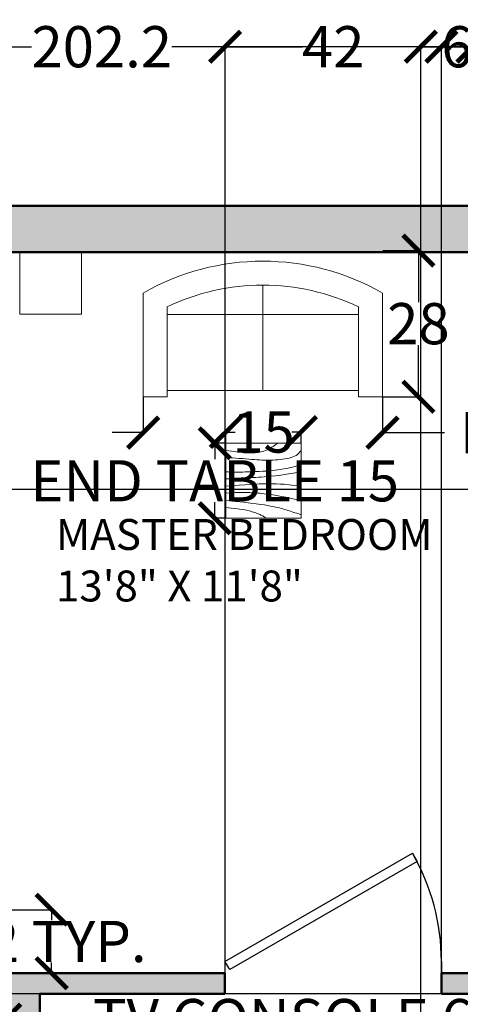
# Model space of a CAD drawing. Units: inches. Extents: x -30 to 744, y -375 to 57.
# Tile 4 of 8: x 116 to 202, y -134 to 57. Entities that reach past the tile are written whole.
import ezdxf

# ---------------------------------------------------------------- set-up
doc = ezdxf.new("R2010")
doc.units = ezdxf.units.IN
doc.header["$MEASUREMENT"] = 0
for name, color, linetype, lineweight in [('A-ANNO-DIMS', 2, 'Continuous', 18), ('A-AREA-IDEN', 7, 'Continuous', 25), ('A-DOOR', 3, 'Continuous', 25), ('A-FURN', 8, 'Continuous', 18), ('A-WALL', 7, 'Continuous', 50)]:
    doc.layers.add(name, color=color, linetype=linetype, lineweight=lineweight)
doc.layers.add('A-WALL-PATT', color=251, linetype='Continuous', lineweight=13, true_color=0x636466)
doc.styles.get("Standard").update_dxf_attribs({"font": 'arial.ttf'})
doc.dimstyles.get("Standard").update_dxf_attribs({"dimtxt": 8, "dimasz": 6, "dimexe": 0.18, "dimexo": 0.0625, "dimgap": 0.09, "dimtad": 0, "dimtih": 1, "dimtoh": 1, "dimdec": 0, "dimzin": 0, "dimdsep": 46, "dimlunit": 4, "dimtxsty": 'Standard', "dimblk": 'ARCHTICK', "dimcen": 0.09, "dimadec": 0, "dimazin": 0, "dimtfac": 1, "dimtdec": 0, "dimtofl": 0, "dimtmove": 0, "dimatfit": 1, "dimldrblk": 'ARCHTICK', "dimfxl": 1, "dimtolj": 1, "dimtzin": 0, "dimarcsym": 0})

# ---------------------------------------------------------------- blocks, each defined once
blk = doc.blocks.new('*U2')
for p, q in [((0, 0), (0, -6)), ((40, 0), (40, -6))]:
    blk.add_line(p, q)
blk.add_lwpolyline([(0, 0), (34.64, 20), (35.52, 18.48), (0.87, -1.52)], close=True)
blk.add_arc((0, 0), 40, 0, 30)
blk = doc.blocks.new('Table - Square Woodgrain 42 x 42 in.')
blk.add_line((0, -42), (42, -42))
for points in [[(0, -4), (1.704, -4.2172), (3.2358, -4.4188), (4.615, -4.604), (5.8615, -4.7721), (6.9951, -4.9224), (8.0357, -5.0541), (9.0031, -5.1667), (9.9171, -5.2594), (10.7951, -5.3316), (11.6445, -5.3836), (12.4702, -5.4157), (13.277, -5.4283), (14.0698, -5.4217), (14.8535, -5.3964), (15.6331, -5.3526), (16.4133, -5.2908), (17.1986, -5.2103), (17.9913, -5.1062), (18.793, -4.9727), (19.6056, -4.8038), (20.4307, -4.5937), (21.2701, -4.3365), (22.1256, -4.0262), (22.9989, -3.6571), (23.888, -3.2272), (24.7756, -2.7516), (25.6408, -2.2491), (26.4624, -1.7387), (27.2195, -1.2395), (27.891, -0.7703), (28.456, -0.3501), (28.8934, 0.002)], [(0, -42), (0, 0), (42, 0), (42, -42)], [(0, -8), (1.8203, -8.1001), (3.6741, -8.2149), (5.5411, -8.3408), (7.4011, -8.4741), (9.2339, -8.6112), (11.0193, -8.7484), (12.7371, -8.8821), (14.3671, -9.0086), (15.8954, -9.1246), (17.3337, -9.2278), (18.6997, -9.3159), (20.0116, -9.387), (21.2871, -9.4389), (22.5442, -9.4696), (23.8008, -9.477), (25.0749, -9.459), (26.3791, -9.4137), (27.7049, -9.3403), (29.0383, -9.2382), (30.3655, -9.1068), (31.6728, -8.9455), (32.9461, -8.7535), (34.1717, -8.5304), (35.3358, -8.2756), (36.4268, -7.9863), (37.443, -7.6521), (38.3849, -7.2603), (39.253, -6.7986), (40.048, -6.2542), (40.7705, -5.6147), (41.421, -4.8674), (42, -4)], [(42, -12), (39.1784, -12.8621), (36.4519, -13.5654), (33.8246, -14.1294), (31.3004, -14.5731), (28.8832, -14.9161), (26.577, -15.1775), (24.3858, -15.3768), (22.3136, -15.5332), (20.3622, -15.6632), (18.5254, -15.7718), (16.7947, -15.8612), (15.1618, -15.9338), (13.6183, -15.9916), (12.1558, -16.0369), (10.7659, -16.0718), (9.4403, -16.0987), (8.1703, -16.1191), (6.9461, -16.1325), (5.7577, -16.1377), (4.595, -16.1335), (3.4479, -16.1188), (2.3064, -16.0924), (1.1604, -16.0532), (0, -16)], [(42, -16), (37.6529, -16.7365), (33.8802, -17.329), (30.6179, -17.7961), (27.8015, -18.1561), (25.3668, -18.4275), (23.2497, -18.6288), (21.3859, -18.7785), (19.7111, -18.8949), (18.1693, -18.9939), (16.7375, -19.0795), (15.401, -19.1534), (14.1449, -19.217), (12.9544, -19.2717), (11.8148, -19.3191), (10.7113, -19.3606), (9.6291, -19.3976), (8.5534, -19.4323), (7.47, -19.4689), (6.3643, -19.5122), (5.222, -19.5672), (4.0288, -19.6386), (2.7703, -19.7313), (1.4321, -19.8501), (0, -20)], [(0, -24), (3.9243, -23.6805), (7.4766, -23.4138), (10.6891, -23.1954), (13.5943, -23.0205), (16.2247, -22.8847), (18.6125, -22.7832), (20.7903, -22.7116), (22.7903, -22.6651), (24.6563, -22.642), (26.4764, -22.6507), (28.35, -22.7024), (30.3766, -22.8084), (32.6555, -22.98), (35.2861, -23.2283), (38.3678, -23.5645), (42, -24)], [(42, -32), (37.392, -31.017), (33.4585, -30.2231), (30.1291, -29.5949), (27.3334, -29.109), (25.0009, -28.742), (23.0612, -28.4707), (21.4439, -28.2716), (20.0786, -28.1215), (18.8998, -28.0002), (17.8609, -27.9014), (16.9206, -27.8219), (16.0371, -27.7588), (15.1691, -27.709), (14.2748, -27.6693), (13.3128, -27.6368), (12.2415, -27.6083), (11.0295, -27.5824), (9.6867, -27.5643), (8.233, -27.5608), (6.6884, -27.5787), (5.0728, -27.6248), (3.4062, -27.7058), (1.7086, -27.8286), (0, -28)], [(0, -32), (5.4026, -32.5358), (9.9494, -33.019), (13.7424, -33.4553), (16.8834, -33.8505), (19.4743, -34.2106), (21.6171, -34.5413), (23.4136, -34.8486), (24.9657, -35.1382), (26.3614, -35.4156), (27.6332, -35.6841), (28.7995, -35.9467), (29.8788, -36.2064), (30.8897, -36.4661), (31.8507, -36.7288), (32.7802, -36.9973), (33.6968, -37.2747), (34.6175, -37.5635), (35.5531, -37.8651), (36.5128, -38.1805), (37.506, -38.5108), (38.5421, -38.8568), (39.6302, -39.2197), (40.7797, -39.6004), (42, -40)], [(0, -36), (3.0098, -36.2857), (5.5354, -36.5643), (7.6368, -36.8359), (9.374, -37.1009), (10.807, -37.3597), (11.9957, -37.6126), (13.0002, -37.8599), (13.8804, -38.102), (14.6874, -38.3393), (15.4365, -38.5729), (16.1338, -38.8041), (16.7858, -39.0341), (17.3987, -39.264), (17.9787, -39.4952), (18.5322, -39.7288), (19.0655, -39.9662), (19.5832, -40.2081), (20.0842, -40.4544), (20.5657, -40.7046), (21.0249, -40.9581), (21.459, -41.2144), (21.8653, -41.4731), (22.2409, -41.7335), (22.5831, -41.9951)]]:
    blk.add_lwpolyline(points)
blk = doc.blocks.new('Sofa - Roundback Loveseat 5 ft.')
for p, q in [((0, -32.44198), (0, -5.99998)), ((-24, -33.99998), (-24, -11.46958)), ((24.00004, -33.99998), (24.00004, -11.46958)), ((-23.9998, -13.38178), (23.99986, -13.38178)), ((-24, -32.44198), (24.00004, -32.44198))]:
    blk.add_line(p, q)
for points in [[(-24, -33.99998), (-30, -33.99998), (-30, -7.99998)], [(30.00004, -7.99998), (30.00004, -33.99998), (24.00004, -33.99998)]]:
    blk.add_lwpolyline(points)
for centre, radius, start, end in [((0, -60.24998), 60.24998, 60.13715, 119.8628), ((0, -61.38438), 55.38444, 64.32083, 115.6792)]:
    blk.add_arc(centre, radius, start, end)
blk = doc.blocks.new('NIGHTSTAND-12IN')
blk.add_lwpolyline([(0, 12), (0, 0), (12, 0), (12, 12)], close=True)
blk = doc.blocks.new('_ArchTick')
at = {"color": 0, "linetype": 'ByBlock', "const_width": 0.15}
blk.add_lwpolyline([(-0.5, -0.5), (0.5, 0.5)], dxfattribs=at)
blk = doc.blocks.new('*D44')
at = {"layer": 'A-ANNO-DIMS', "color": 0, "lineweight": -2, "transparency": 16777216}
for p, q in [((53.6, -128.37), (53.6, -137.48)), ((113.6, -128.37), (113.6, -137.48)), ((53.6, -137.3), (47.6, -137.3)), ((113.6, -137.3), (125.6, -137.3))]:
    blk.add_line(p, q, dxfattribs=at)
at = {"layer": 'Defpoints', "color": 0, "transparency": 16777216}
for p in [(53.6, -128.3), (113.6, -128.3), (113.6, -137.3)]:
    blk.add_point(p, dxfattribs=at)
at = {"layer": 'A-ANNO-DIMS', "color": 0, "lineweight": -2, "transparency": 16777216, "xscale": 6, "yscale": 6, "zscale": 6}
blk.add_blockref('_ArchTick', (53.6, -137.3), dxfattribs=at)
at = {"layer": 'A-ANNO-DIMS', "color": 0, "lineweight": -2, "transparency": 16777216, "xscale": 6, "yscale": 6, "zscale": 6, "rotation": 180}
blk.add_blockref('_ArchTick', (113.6, -137.3), dxfattribs=at)
at = {"layer": 'A-ANNO-DIMS', "color": 0, "transparency": 16777216, "insert": (182.83, -137.3), "char_height": 8, "attachment_point": 5}
blk.add_mtext('\\A1;TV CONSOLE 60 TYP.', dxfattribs=at)
blk = doc.blocks.new('*D45')
at = {"layer": 'A-ANNO-DIMS', "color": 0, "lineweight": -2, "transparency": 16777216}
for p, q in [((113.66, -115.96), (122.78, -115.96)), ((122.6, -115.96), (122.6, -118.02)), ((122.6, -128.3), (122.6, -126.24)), ((113.66, -128.3), (122.78, -128.3))]:
    blk.add_line(p, q, dxfattribs=at)
at = {"layer": 'Defpoints', "color": 0, "transparency": 16777216}
for p in [(113.6, -115.96), (122.6, -115.96), (113.6, -128.3)]:
    blk.add_point(p, dxfattribs=at)
at = {"layer": 'A-ANNO-DIMS', "color": 0, "lineweight": -2, "transparency": 16777216, "xscale": 6, "yscale": 6, "zscale": 6}
for p, rotation in [((122.6, -115.96), 90), ((122.6, -128.3), 270)]:
    blk.add_blockref('_ArchTick', p, dxfattribs=dict(at, rotation=rotation))
at = {"layer": 'A-ANNO-DIMS', "color": 0, "transparency": 16777216, "insert": (122.6, -122.13), "char_height": 8, "attachment_point": 5}
blk.add_mtext('\\A1;12 TYP.', dxfattribs=at)
blk = doc.blocks.new('*D54')
at = {"layer": 'A-ANNO-DIMS', "color": 0, "lineweight": -2, "transparency": 16777216}
for p, q in [((156.36, -25.4), (154.06, -25.4)), ((154.24, -25.4), (154.24, -28.5)), ((154.24, -39.96), (154.24, -36.85)), ((156.36, -39.96), (154.06, -39.96))]:
    blk.add_line(p, q, dxfattribs=at)
at = {"layer": 'Defpoints', "color": 0, "transparency": 16777216}
for p in [(154.24, -25.4), (156.42, -25.4), (156.42, -39.96)]:
    blk.add_point(p, dxfattribs=at)
at = {"layer": 'A-ANNO-DIMS', "color": 0, "lineweight": -2, "transparency": 16777216, "xscale": 6, "yscale": 6, "zscale": 6}
for p, rotation in [((154.24, -25.4), 90), ((154.24, -39.96), 270)]:
    blk.add_blockref('_ArchTick', p, dxfattribs=dict(at, rotation=rotation))
at = {"layer": 'A-ANNO-DIMS', "color": 0, "transparency": 16777216, "insert": (154.24, -32.68), "char_height": 8, "attachment_point": 5}
blk.add_mtext('\\A1;END TABLE 15', dxfattribs=at)
blk = doc.blocks.new('*D55')
at = {"layer": 'A-ANNO-DIMS', "color": 0, "lineweight": -2, "transparency": 16777216}
for p, q in [((156.42, -25.33), (156.42, -23.03)), ((156.42, -23.21), (158.23, -23.21)), ((170.99, -23.21), (169.18, -23.21)), ((170.99, -25.33), (170.99, -23.03))]:
    blk.add_line(p, q, dxfattribs=at)
at = {"layer": 'Defpoints', "color": 0, "transparency": 16777216}
for p in [(170.99, -23.21), (156.42, -25.4), (170.99, -25.4)]:
    blk.add_point(p, dxfattribs=at)
at = {"layer": 'A-ANNO-DIMS', "color": 0, "lineweight": -2, "transparency": 16777216, "xscale": 6, "yscale": 6, "zscale": 6, "rotation": 180}
blk.add_blockref('_ArchTick', (156.42, -23.21), dxfattribs=at)
at = {"layer": 'A-ANNO-DIMS', "color": 0, "lineweight": -2, "transparency": 16777216, "xscale": 6, "yscale": 6, "zscale": 6}
blk.add_blockref('_ArchTick', (170.99, -23.21), dxfattribs=at)
at = {"layer": 'A-ANNO-DIMS', "color": 0, "transparency": 16777216, "insert": (163.71, -23.21), "char_height": 8, "attachment_point": 5}
blk.add_mtext('\\A1;15', dxfattribs=at)
blk = doc.blocks.new('*D56')
at = {"layer": 'A-ANNO-DIMS', "color": 0, "lineweight": -2, "transparency": 16777216}
for p, q in [((140.35, -16.43), (140.35, -23.51)), ((186.8, -16.43), (186.8, -23.51)), ((140.35, -23.33), (134.35, -23.33)), ((186.8, -23.33), (198.8, -23.33))]:
    blk.add_line(p, q, dxfattribs=at)
at = {"layer": 'Defpoints', "color": 0, "transparency": 16777216}
for p in [(140.35, -16.36), (186.8, -16.36), (186.8, -23.33)]:
    blk.add_point(p, dxfattribs=at)
at = {"layer": 'A-ANNO-DIMS', "color": 0, "lineweight": -2, "transparency": 16777216, "xscale": 6, "yscale": 6, "zscale": 6}
blk.add_blockref('_ArchTick', (140.35, -23.33), dxfattribs=at)
at = {"layer": 'A-ANNO-DIMS', "color": 0, "lineweight": -2, "transparency": 16777216, "xscale": 6, "yscale": 6, "zscale": 6, "rotation": 180}
blk.add_blockref('_ArchTick', (186.8, -23.33), dxfattribs=at)
at = {"layer": 'A-ANNO-DIMS', "color": 0, "transparency": 16777216, "insert": (235.5, -23.33), "char_height": 8, "attachment_point": 5}
blk.add_mtext('\\A1;LOVESEAT 46', dxfattribs=at)
blk = doc.blocks.new('*D57')
at = {"layer": 'A-ANNO-DIMS', "color": 0, "lineweight": -2, "transparency": 16777216}
for p, q in [((186.86, 12.03), (193.95, 12.03)), ((193.77, 12.03), (193.77, 2.01)), ((193.77, -16.36), (193.77, -6.34)), ((186.86, -16.36), (193.95, -16.36))]:
    blk.add_line(p, q, dxfattribs=at)
at = {"layer": 'Defpoints', "color": 0, "transparency": 16777216}
for p in [(186.8, 12.03), (193.77, 12.03), (186.8, -16.36)]:
    blk.add_point(p, dxfattribs=at)
at = {"layer": 'A-ANNO-DIMS', "color": 0, "lineweight": -2, "transparency": 16777216, "xscale": 6, "yscale": 6, "zscale": 6}
for p, rotation in [((193.77, 12.03), 90), ((193.77, -16.36), 270)]:
    blk.add_blockref('_ArchTick', p, dxfattribs=dict(at, rotation=rotation))
at = {"layer": 'A-ANNO-DIMS', "color": 0, "transparency": 16777216, "insert": (193.77, -2.17), "char_height": 8, "attachment_point": 5}
blk.add_mtext('\\A1;28', dxfattribs=at)
blk = doc.blocks.new('*D63')
at = {"layer": 'A-ANNO-DIMS', "color": 0, "lineweight": -2, "transparency": 16777216}
for p, q in [((542.17, -132.3), (-16.61, -132.3)), ((-16.43, -132.3), (-16.43, -157.12)), ((-16.43, -190.3), (-16.43, -165.47)), ((542.17, -190.3), (-16.61, -190.3))]:
    blk.add_line(p, q, dxfattribs=at)
at = {"layer": 'Defpoints', "color": 0, "transparency": 16777216}
for p in [(-16.43, -132.3), (542.24, -132.3), (542.24, -190.3)]:
    blk.add_point(p, dxfattribs=at)
at = {"layer": 'A-ANNO-DIMS', "color": 0, "lineweight": -2, "transparency": 16777216, "xscale": 6, "yscale": 6, "zscale": 6}
for p, rotation in [((-16.43, -132.3), 90), ((-16.43, -190.3), 270)]:
    blk.add_blockref('_ArchTick', p, dxfattribs=dict(at, rotation=rotation))
at = {"layer": 'A-ANNO-DIMS', "color": 0, "transparency": 16777216, "insert": (-16.43, -161.3), "char_height": 8, "attachment_point": 5}
blk.add_mtext('\\A1;58', dxfattribs=at)
blk = doc.blocks.new('*D66')
at = {"layer": 'A-ANNO-DIMS', "color": 0, "lineweight": -2, "transparency": 16777216}
for p, q in [((156.24, -128.23), (156.24, 51.78)), ((198.24, -128.23), (198.24, 51.78)), ((156.24, 51.6), (171.3, 51.6)), ((198.24, 51.6), (183.18, 51.6))]:
    blk.add_line(p, q, dxfattribs=at)
at = {"layer": 'Defpoints', "color": 0, "transparency": 16777216}
for p in [(198.24, 51.6), (156.24, -128.3), (198.24, -128.3)]:
    blk.add_point(p, dxfattribs=at)
at = {"layer": 'A-ANNO-DIMS', "color": 0, "lineweight": -2, "transparency": 16777216, "xscale": 6, "yscale": 6, "zscale": 6, "rotation": 180}
blk.add_blockref('_ArchTick', (156.24, 51.6), dxfattribs=at)
at = {"layer": 'A-ANNO-DIMS', "color": 0, "lineweight": -2, "transparency": 16777216, "xscale": 6, "yscale": 6, "zscale": 6}
blk.add_blockref('_ArchTick', (198.24, 51.6), dxfattribs=at)
at = {"layer": 'A-ANNO-DIMS', "color": 0, "transparency": 16777216, "insert": (177.24, 51.6), "char_height": 8, "attachment_point": 5}
blk.add_mtext('\\A1;42', dxfattribs=at)
blk = doc.blocks.new('*D69')
at = {"layer": 'A-ANNO-DIMS', "color": 0, "lineweight": -2, "transparency": 16777216}
for p, q in [((31.24, 20.77), (31.24, 51.78)), ((233.43, 20.77), (233.43, 51.78)), ((31.24, 51.6), (118.72, 51.6)), ((233.43, 51.6), (145.95, 51.6))]:
    blk.add_line(p, q, dxfattribs=at)
at = {"layer": 'Defpoints', "color": 0, "transparency": 16777216}
for p in [(233.43, 51.6), (31.24, 20.7), (233.43, 20.7)]:
    blk.add_point(p, dxfattribs=at)
at = {"layer": 'A-ANNO-DIMS', "color": 0, "lineweight": -2, "transparency": 16777216, "xscale": 6, "yscale": 6, "zscale": 6, "rotation": 180}
blk.add_blockref('_ArchTick', (31.24, 51.6), dxfattribs=at)
at = {"layer": 'A-ANNO-DIMS', "color": 0, "lineweight": -2, "transparency": 16777216, "xscale": 6, "yscale": 6, "zscale": 6}
blk.add_blockref('_ArchTick', (233.43, 51.6), dxfattribs=at)
at = {"layer": 'A-ANNO-DIMS', "color": 0, "transparency": 16777216, "insert": (132.33, 51.6), "char_height": 8, "attachment_point": 5}
blk.add_mtext('\\A1;202.2', dxfattribs=at)
blk = doc.blocks.new('*D73')
at = {"layer": 'A-ANNO-DIMS', "color": 0, "lineweight": -2, "transparency": 16777216}
for p, q in [((194.24, -330.23), (194.24, 51.78)), ((230.24, -330.23), (230.24, 51.78)), ((194.24, 51.6), (206.42, 51.6)), ((230.24, 51.6), (218.05, 51.6))]:
    blk.add_line(p, q, dxfattribs=at)
at = {"layer": 'Defpoints', "color": 0, "transparency": 16777216}
for p in [(230.24, 51.6), (194.24, -330.3), (230.24, -330.3)]:
    blk.add_point(p, dxfattribs=at)
at = {"layer": 'A-ANNO-DIMS', "color": 0, "lineweight": -2, "transparency": 16777216, "xscale": 6, "yscale": 6, "zscale": 6, "rotation": 180}
blk.add_blockref('_ArchTick', (194.24, 51.6), dxfattribs=at)
at = {"layer": 'A-ANNO-DIMS', "color": 0, "lineweight": -2, "transparency": 16777216, "xscale": 6, "yscale": 6, "zscale": 6}
blk.add_blockref('_ArchTick', (230.24, 51.6), dxfattribs=at)
at = {"layer": 'A-ANNO-DIMS', "color": 0, "transparency": 16777216, "insert": (212.24, 51.6), "char_height": 8, "attachment_point": 5}
blk.add_mtext('\\A1;36', dxfattribs=at)
blk = doc.blocks.new('*D75')
at = {"layer": 'A-ANNO-DIMS', "color": 0, "lineweight": -2, "transparency": 16777216}
for p, q in [((40.3, 11.7), (662.32, 11.7)), ((662.14, 11.7), (662.14, -7.12)), ((662.14, -34.3), (662.14, -15.47)), ((40.3, -34.3), (662.32, -34.3))]:
    blk.add_line(p, q, dxfattribs=at)
at = {"layer": 'Defpoints', "color": 0, "transparency": 16777216}
for p in [(40.24, 11.7), (662.14, 11.7), (40.24, -34.3)]:
    blk.add_point(p, dxfattribs=at)
at = {"layer": 'A-ANNO-DIMS', "color": 0, "lineweight": -2, "transparency": 16777216, "xscale": 6, "yscale": 6, "zscale": 6}
for p, rotation in [((662.14, 11.7), 90), ((662.14, -34.3), 270)]:
    blk.add_blockref('_ArchTick', p, dxfattribs=dict(at, rotation=rotation))
at = {"layer": 'A-ANNO-DIMS', "color": 0, "transparency": 16777216, "insert": (662.14, -11.3), "char_height": 8, "attachment_point": 5}
blk.add_mtext('\\A1;46', dxfattribs=at)
blk = doc.blocks.new('*D86')
at = {"layer": 'A-ANNO-DIMS', "color": 0, "lineweight": -2, "transparency": 16777216}
for p, q in [((198.24, -128.23), (198.24, 51.78)), ((204.24, -128.23), (204.24, 51.78)), ((198.24, 51.6), (198.5, 51.6)), ((204.24, 51.6), (203.97, 51.6))]:
    blk.add_line(p, q, dxfattribs=at)
at = {"layer": 'Defpoints', "color": 0, "transparency": 16777216}
for p in [(204.24, 51.6), (198.24, -128.3), (204.24, -128.3)]:
    blk.add_point(p, dxfattribs=at)
at = {"layer": 'A-ANNO-DIMS', "color": 0, "lineweight": -2, "transparency": 16777216, "xscale": 6, "yscale": 6, "zscale": 6, "rotation": 180}
blk.add_blockref('_ArchTick', (198.24, 51.6), dxfattribs=at)
at = {"layer": 'A-ANNO-DIMS', "color": 0, "lineweight": -2, "transparency": 16777216, "xscale": 6, "yscale": 6, "zscale": 6}
blk.add_blockref('_ArchTick', (204.24, 51.6), dxfattribs=at)
at = {"layer": 'A-ANNO-DIMS', "color": 0, "transparency": 16777216, "insert": (201.24, 51.6), "char_height": 8, "attachment_point": 5}
blk.add_mtext('\\A1;6', dxfattribs=at)

msp = doc.modelspace()

# ---------------------------------------------------------------- hatches: boundary and pattern name
at = {"layer": 'A-WALL-PATT'}
h = msp.add_hatch(color=256, dxfattribs=at)
h.dxf.hatch_style = 1
h.paths.add_polyline_path([(40.2356, 11.7031), (204.2356, 11.7031), (204.2356, -24.2969), (208.2356, -24.2969), (208.2356, 11.7031), (233.4275, 11.7031), (233.4275, 20.7031), (31.2356, 20.7031), (31.2356, -34.2969), (40.2356, -34.2969)])
h.paths.add_polyline_path([(40.2356, -82.2969), (31.2356, -82.2969), (31.2356, -132.2969), (40.2356, -132.2969), (51.0767, -132.2969), (111.3137, -132.2969), (111.3137, -143.2969), (120.3137, -143.2969), (120.3137, -132.2969), (156.2356, -132.2969), (156.2356, -128.2969), (113.6001, -128.2969), (113.6001, -128.3034), (53.6001, -128.3034), (40.2356, -128.2969)])
h.paths.add_polyline_path([(302.4681, 20.7031), (257.4275, 20.7031), (257.4275, 11.7031), (286.2356, 11.7031), (286.2356, -60.2969), (208.2356, -60.2969), (208.2356, -54.2969), (204.2356, -54.2969), (204.2356, -64.2969), (208.2356, -64.2969), (286.2356, -64.2969), (286.2356, -128.2969), (264.8954, -128.2969), (208.2356, -128.2969), (204.2356, -128.2969), (198.2356, -128.2969), (198.2356, -132.2969), (290.2356, -132.2969), (290.2356, -128.2969), (290.2356, 11.7031), (302.4681, 11.7031)])
h.paths.add_polyline_path([(405.515, 20.7031), (350.4681, 20.7031), (350.4681, 11.7031), (362.2356, 11.7031), (362.2356, -34.2969), (366.2356, -34.2969), (366.2356, 11.7031), (405.515, 11.7031)])
h.paths.add_polyline_path([(530.2713, 20.7031), (453.515, 20.7031), (453.515, 11.7031), (486.2356, 11.7031), (486.2356, -128.2969), (448.2356, -128.2969), (448.2356, -132.2969), (486.2356, -132.2969), (490.2356, -132.2969), (496.2356, -132.2969), (496.2356, -128.2969), (490.2356, -128.2969), (490.2356, 11.7031), (530.2713, 11.7031)])
h.paths.add_polyline_path([(631.2356, 20.7031), (578.2713, 20.7031), (578.2713, 11.7031), (622.2356, 11.7031), (622.2356, -37.4001), (631.2356, -37.4001)])
h.paths.add_polyline_path([(631.2356, -85.4001), (622.2356, -85.4001), (622.2356, -91.4001), (622.2356, -103.4001), (622.2356, -128.2969), (538.2356, -128.2969), (538.2356, -132.2969), (538.2356, -154.2969), (542.2356, -154.2969), (542.2356, -132.2969), (575.1375, -132.2969), (585.6313, -131.9348), (585.6438, -132.2969), (622.2356, -132.2969), (622.2356, -147.2969), (631.2356, -147.2969)])
h.paths.add_polyline_path([(631.2356, -171.2969), (622.2356, -171.2969), (622.2356, -185.4028), (622.2356, -186.2969), (622.2356, -190.2969), (542.2356, -190.2969), (542.2356, -184.2969), (538.2356, -184.2969), (538.2356, -190.2969), (538.2356, -194.2969), (622.2356, -194.2969), (622.2356, -237.4632), (631.2356, -237.4632)])
h.paths.add_polyline_path([(631.2356, -285.4632), (622.2356, -285.4632), (622.2356, -330.2969), (490.2356, -330.2969), (490.2356, -194.2969), (494.2356, -194.2969), (495.2356, -194.2969), (495.2356, -190.2969), (494.2356, -190.2969), (490.2356, -190.2969), (486.2356, -190.2969), (366.2356, -190.2969), (366.2356, -194.2969), (486.2356, -194.2969), (486.2356, -330.2969), (426.2356, -330.2969), (426.2356, -339.2969), (631.2356, -339.2969)])
h.paths.add_polyline_path([(378.2356, -330.2969), (318.2356, -330.2969), (318.2356, -194.2969), (324.2356, -194.2969), (324.2356, -190.2969), (318.2356, -190.2969), (314.2356, -190.2969), (314.2356, -194.2969), (314.2356, -330.2969), (278.2356, -330.2969), (278.2356, -339.2969), (378.2356, -339.2969)])
h.paths.add_polyline_path([(190.2356, -330.2969), (40.2356, -330.2969), (40.2356, -318.2969), (31.2356, -318.2969), (31.2356, -330.2969), (31.2356, -339.2969), (190.2356, -339.2969)])
h.paths.add_polyline_path([(230.2356, -330.2969), (194.2356, -330.2969), (194.2356, -194.2969), (194.2356, -190.2969), (190.2356, -190.2969), (184.2356, -190.2969), (184.2356, -194.2969), (190.2356, -194.2969), (190.2356, -339.2969), (230.2356, -339.2969)])
h.paths.add_polyline_path([(142.2356, -190.2969), (120.3137, -190.2969), (120.3137, -184.2969), (116.3137, -184.2969), (111.3137, -184.2969), (111.3137, -190.2969), (40.2356, -190.2969), (31.2356, -190.2969), (31.2356, -194.2969), (31.2356, -206.2969), (40.2356, -206.2969), (40.2356, -194.2969), (142.2356, -194.2969)])

# ---------------------------------------------------------------- linework, layer by layer
at = {"layer": 'A-WALL'}
for p, q in [((40.2356, 11.7031), (204.2356, 11.7031)), ((40.2356, -128.2969), (156.2356, -128.2969)), ((156.2356, -132.2969), (156.2356, -128.2969)), ((198.2356, -132.2969), (198.2356, -128.2969)), ((198.2356, -128.2969), (204.2356, -128.2969)), ((120.3137, -143.2969), (120.3137, -132.2969)), ((120.3137, -132.2969), (156.2356, -132.2969)), ((198.2356, -132.2969), (290.2356, -132.2969))]:
    msp.add_line(p, q, dxfattribs=at)
msp.add_lwpolyline([(31.2356, -132.2969), (31.2356, 20.7031), (631.2356, 20.7031), (631.2356, -339.2969), (190.2356, -339.2969)], dxfattribs=at)

# ---------------------------------------------------------------- block references
at = {"layer": 'A-DOOR', "xscale": 1.05, "yscale": 1.05, "zscale": 1.05}
msp.add_blockref('*U2', (156.2356, -125.9969), dxfattribs=at)
at = {"layer": 'A-FURN', "rotation": 90.00000000000018}
msp.add_blockref('NIGHTSTAND-12IN', (128.4058, -0.2964), dxfattribs=at)
at = {"layer": 'A-FURN'}
for name, p, xscale, yscale, zscale in [('Sofa - Roundback Loveseat 5 ft.', (163.5734, 9.9606), 0.774270265219057, 0.774270265219057, 0.774270265219057), ('Table - Square Woodgrain 42 x 42 in.', (156.4245, -25.3963), 0.3467624583282872, 0.3467624583282872, 0.3467624583282872)]:
    msp.add_blockref(name, p, dxfattribs=dict(at, xscale=xscale, yscale=yscale, zscale=zscale))

# ---------------------------------------------------------------- texts
at = {"layer": 'A-AREA-IDEN', "insert": (123.4304, -40.1069), "char_height": 6, "attachment_point": 1}
msp.add_mtext_dynamic_manual_height_columns('MASTER BEDROOM\\P13\'8" X 11\'8"', width=80.805182, gutter_width=1, heights=[0], dxfattribs=at)

# ---------------------------------------------------------------- dimensions: what is measured, and where the dimension line sits
at = {"layer": 'A-ANNO-DIMS'}
for base, p1, p2, override, picture, middle in [((233.4275, 51.6031), (31.2356, 20.7031), (233.4275, 20.7031), {"dimdec": 1, "dimlfac": 1, "dimrnd": 0, "dimzin": 0, "dimdsep": 46, "dimlunit": 2}, '*D69', (132.3315, 51.6031)), ((198.2356, 51.6031), (156.2356, -128.2969), (198.2356, -128.2969), {"dimdec": 0, "dimlfac": 1, "dimrnd": 0, "dimzin": 0, "dimdsep": 46, "dimlunit": 2}, '*D66', (177.2356, 51.6031)), ((230.2356, 51.6031), (194.2356, -330.2969), (230.2356, -330.2969), {"dimdec": 0, "dimlfac": 1, "dimrnd": 0, "dimzin": 0, "dimdsep": 46, "dimlunit": 2}, '*D73', (212.2356, 51.6031)), ((204.2356, 51.6031), (198.2356, -128.2969), (204.2356, -128.2969), {"dimdec": 0, "dimlfac": 1, "dimrnd": 0, "dimzin": 0, "dimdsep": 46, "dimlunit": 2}, '*D86', (201.2356, 51.6031)), ((170.9885, -23.2109), (156.4245, -25.3956), (170.9885, -25.3956), {"dimdec": 0, "dimlfac": 1, "dimrnd": 0, "dimzin": 0, "dimdsep": 46, "dimlunit": 2}, '*D55', (163.7065, -23.2109))]:
    dim = msp.add_linear_dim(base=base, p1=p1, p2=p2, dimstyle='Standard', override=override, dxfattribs=at)
    dim.commit()
    dim.dimension.update_dxf_attribs({"geometry": picture, "text_midpoint": middle})
for base, p1, p2, picture, middle in [((193.77, 12.0254), (186.8015, -16.3645), (186.8015, 12.0254), '*D57', (193.77, -2.1696)), ((662.1356, 11.7031), (40.2356, -34.2969), (40.2356, 11.7031), '*D75', (662.1356, -11.2969)), ((-16.4253, -132.2969), (542.2356, -190.2969), (542.2356, -132.2969), '*D63', (-16.4253, -161.2969))]:
    dim = msp.add_linear_dim(base=base, p1=p1, p2=p2, angle=90, dimstyle='Standard', override={"dimdec": 0, "dimlfac": 1, "dimrnd": 0, "dimzin": 0, "dimdsep": 46, "dimlunit": 2}, dxfattribs=at)
    dim.commit()
    dim.dimension.update_dxf_attribs({"geometry": picture, "text_midpoint": middle})
for base, p1, p2, text, picture, middle in [((186.8015, -23.333), (140.3453, -16.3645), (186.8015, -16.3645), 'LOVESEAT <>', '*D56', (235.4973, -23.333)), ((113.6001, -137.3034), (53.6001, -128.3034), (113.6001, -128.3034), 'TV CONSOLE <> TYP.', '*D44', (182.8334, -137.3034))]:
    dim = msp.add_linear_dim(base=base, p1=p1, p2=p2, text=text, dimstyle='Standard', override={"dimdec": 0, "dimlfac": 1, "dimrnd": 0, "dimzin": 0, "dimdsep": 46, "dimlunit": 2}, dxfattribs=at)
    dim.commit()
    dim.dimension.update_dxf_attribs({"geometry": picture, "text_midpoint": middle})
for base, p1, p2, text, picture, middle in [((154.2398, -25.3956), (156.4245, -39.9603), (156.4245, -25.3956), 'END TABLE <>', '*D54', (154.2398, -32.678)), ((122.6001, -115.9579), (113.6001, -128.3034), (113.6001, -115.9579), '<> TYP.', '*D45', (122.6001, -122.1306))]:
    dim = msp.add_linear_dim(base=base, p1=p1, p2=p2, angle=90, text=text, dimstyle='Standard', override={"dimdec": 0, "dimlfac": 1, "dimrnd": 0, "dimzin": 0, "dimdsep": 46, "dimlunit": 2}, dxfattribs=at)
    dim.commit()
    dim.dimension.update_dxf_attribs({"geometry": picture, "text_midpoint": middle})

doc.saveas('drawing.dxf')
